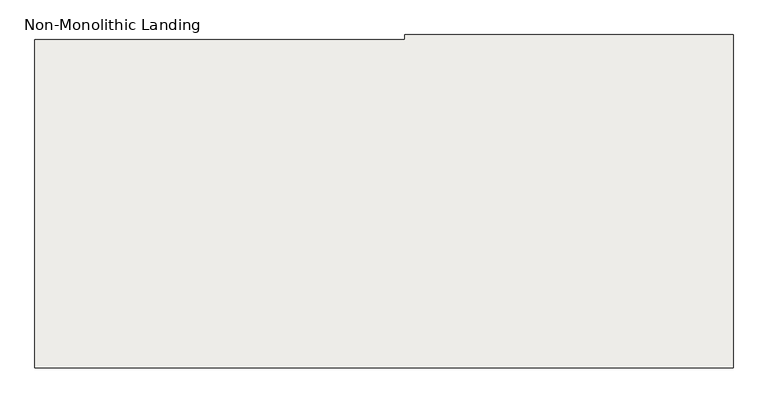
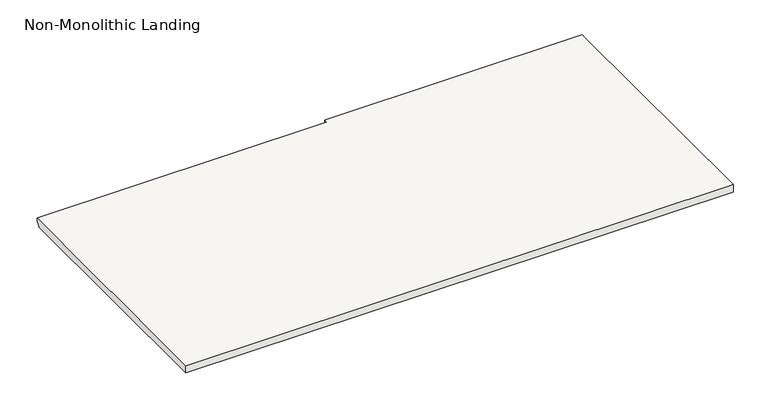
"""IFC4 building model written with IfcOpenShell, lengths in millimetres: slab geometry, Non-Monolithic Landing."""

from ifc_helpers import new_model, si_unit, origin, place, context, project, spatial, faceted_brep, source, transform, mapped, element, save


def non_monolithic_landing_4cda9577(model_context):
    return source(origin(), model_context, "Body", "Brep", [
        faceted_brep([(53660.3072437, 30926.7590238, 2089.15), (53660.3072437, 30952.1590238, 2114.55), (55336.7072437, 30952.1590238, 2114.55), (55336.7072437, 30926.7590238, 2089.15), (53660.3072437, 29275.7590238, 2133.6), (57222.9312819, 29275.7590238, 2133.6), (57222.9312819, 30952.1590238, 2133.6), (57222.9312819, 30977.5590238, 2133.6), (55546.5312819, 30977.5590238, 2133.6), (55546.5312819, 30952.1590238, 2133.6), (53660.3072437, 30952.1590238, 2133.6), (55336.7072437, 30926.7590238, 2082.8), (55336.7072437, 30952.1590238, 2082.8), (55546.5312819, 30952.1590238, 2082.8), (55546.5312819, 30977.5590238, 2082.8), (57222.9312819, 30977.5590238, 2082.8), (57222.9312819, 30952.1590238, 2082.8), (57222.9312819, 29275.7590238, 2082.8), (53660.3072437, 29275.7590238, 2082.8), (53660.3072437, 30926.7590238, 2082.8)], [[[0, 1, 2, 3]], [[4, 5, 6, 7, 8, 9, 10]], [[11, 12, 13, 14, 15, 16, 17, 18, 19]], [[12, 11, 3, 2]], [[11, 19, 0, 3]], [[4, 10, 1, 0, 19, 18]], [[5, 4, 18, 17]], [[6, 5, 17, 16]], [[7, 6, 16, 15]], [[8, 7, 15, 14]], [[9, 8, 14, 13]], [[10, 9, 13, 12, 2, 1]]]),
    ])


if __name__ == "__main__":
    model = new_model("IFC4")
    model_context = context("Model", 3, world=origin())
    ifc_project = project(units=[si_unit("LENGTHUNIT", "METRE", prefix="MILLI")], contexts=[model_context])
    site = spatial("IfcSite", under=ifc_project)
    building = spatial("IfcBuilding", under=site)
    placement = place(None, origin())
    non_monolithic_landing_shape = non_monolithic_landing_4cda9577(model_context)
    element("IfcSlab", 1, ObjectType="Non-Monolithic Landing", at=placement, inside=building, context=model_context, shape_type="MappedRepresentation", body=[
        mapped(non_monolithic_landing_shape, transform((0.0, 0.0, 0.0), x_axis=(1.0, 0.0, 0.0), y_axis=(0.0, 1.0, 0.0), z_axis=(0.0, 0.0, 1.0))),
    ])
    save(model, "model.ifc")
